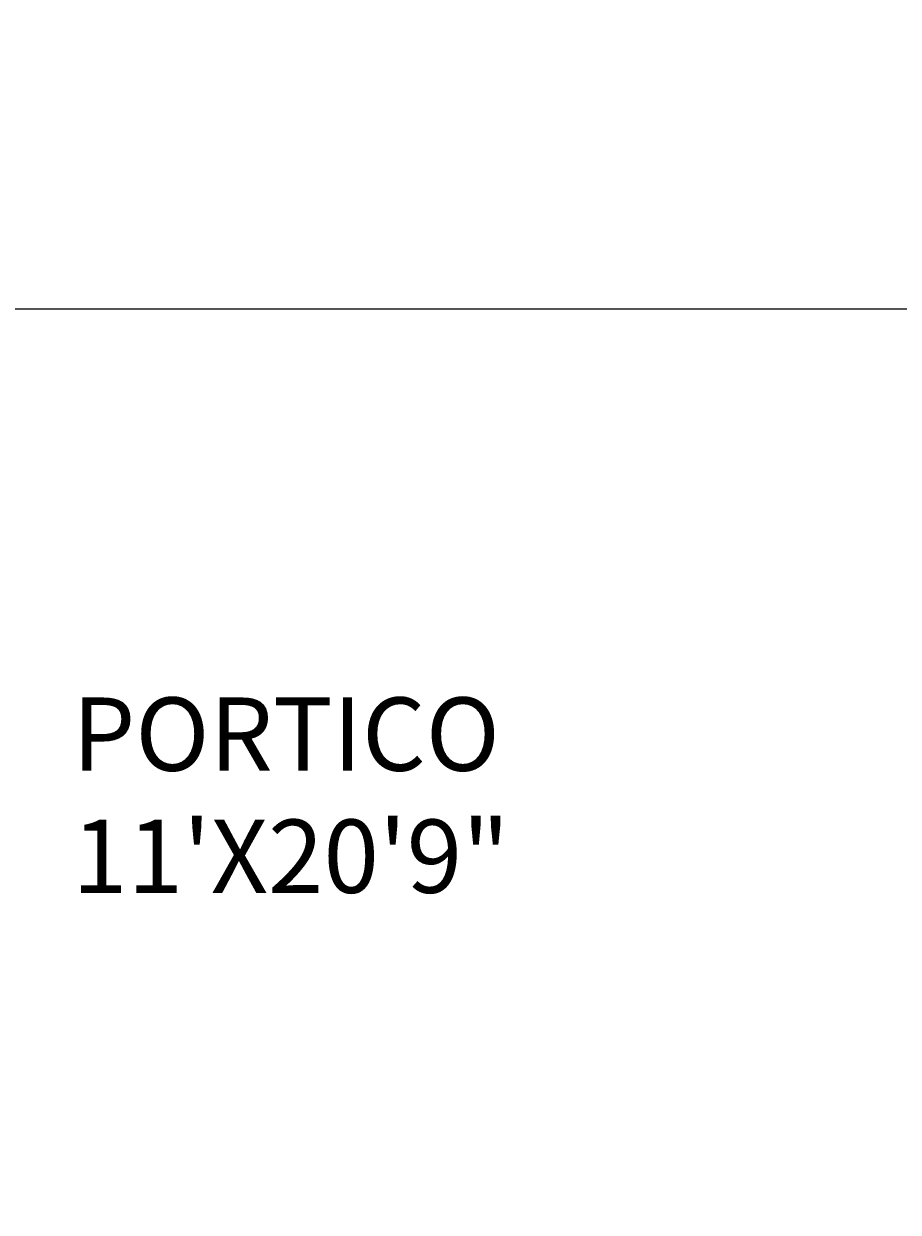
# Model space of a CAD drawing. Units: inches. Extents: x -4347 to -3836, y 955 to 1521.
# Tile 6 of 11: x -4072 to -4001, y 1023 to 1120. Entities that reach past the tile are written whole.
import ezdxf

# ---------------------------------------------------------------- set-up
doc = ezdxf.new("R2010")
doc.units = ezdxf.units.IN
doc.header["$MEASUREMENT"] = 0
doc.layers.add('A-ANNO-DIMS', color=2, linetype='Continuous', lineweight=18)
doc.layers.add('A-AREA-IDEN', color=7, linetype='Continuous', lineweight=18)
doc.styles.get("Standard").update_dxf_attribs({"font": 'arial.ttf'})
doc.dimstyles.get("Standard").update_dxf_attribs({"dimtxt": 0.18, "dimasz": 0.18, "dimexe": 0.18, "dimexo": 0.0625, "dimgap": 0.09, "dimtad": 0, "dimtih": 1, "dimtoh": 1, "dimdec": 0, "dimzin": 0, "dimdsep": 46, "dimlunit": 3, "dimtxsty": 'Standard', "dimcen": 0.09, "dimadec": 0, "dimazin": 0, "dimtfac": 1, "dimtdec": 0, "dimtofl": 0, "dimtmove": 0, "dimatfit": 3, "dimfxl": 1, "dimtolj": 1, "dimtzin": 0, "dimarcsym": 0})

# ---------------------------------------------------------------- blocks, each defined once
blk = doc.blocks.new('*D47')
at = {"layer": 'A-ANNO-DIMS', "color": 0, "lineweight": -2, "transparency": 16777216}
for p, q in [((-4120.58, 1288.726), (-4120.58, 966.959)), ((-3940.58, 1288.726), (-3940.58, 966.959)), ((-4120.4, 967.139), (-4030.97, 967.139)), ((-3940.76, 967.139), (-4030.189, 967.139))]:
    blk.add_line(p, q, dxfattribs=at)
at = {"layer": 'A-ANNO-DIMS', "color": 0, "transparency": 16777216}
for points in [[(-4120.4, 967.169), (-4120.4, 967.109), (-4120.58, 967.139)], [(-3940.76, 967.169), (-3940.76, 967.109), (-3940.58, 967.139)]]:
    blk.add_solid(points, dxfattribs=at)
at = {"layer": 'Defpoints', "color": 0, "transparency": 16777216}
for p in [(-4120.58, 1288.789), (-3940.58, 1288.789), (-3940.58, 967.139)]:
    blk.add_point(p, dxfattribs=at)
at = {"layer": 'A-ANNO-DIMS', "color": 0, "transparency": 16777216, "insert": (-4030.58, 967.139), "char_height": 0.18, "attachment_point": 5}
blk.add_mtext('\\A1;15\'-0"', dxfattribs=at)
blk = doc.blocks.new('*D54')
at = {"layer": 'A-ANNO-DIMS', "color": 0, "lineweight": -2, "transparency": 16777216}
for p, q in [((-3997.757, 1126.789), (-4346.41, 1126.789)), ((-4346.23, 1126.609), (-4346.23, 1111.971)), ((-4346.23, 1096.969), (-4346.23, 1111.607)), ((-3997.757, 1096.789), (-4346.41, 1096.789))]:
    blk.add_line(p, q, dxfattribs=at)
at = {"layer": 'A-ANNO-DIMS', "color": 0, "transparency": 16777216}
for points in [[(-4346.26, 1126.609), (-4346.2, 1126.609), (-4346.23, 1126.789)], [(-4346.26, 1096.969), (-4346.2, 1096.969), (-4346.23, 1096.789)]]:
    blk.add_solid(points, dxfattribs=at)
at = {"layer": 'Defpoints', "color": 0, "transparency": 16777216}
for p in [(-4346.23, 1126.789), (-3997.694, 1126.789), (-3997.694, 1096.789)]:
    blk.add_point(p, dxfattribs=at)
at = {"layer": 'A-ANNO-DIMS', "color": 0, "transparency": 16777216, "insert": (-4346.23, 1111.789), "char_height": 0.18, "attachment_point": 5}
blk.add_mtext('\\A1;2\'-6"', dxfattribs=at)

msp = doc.modelspace()

# ---------------------------------------------------------------- texts
at = {"layer": 'A-AREA-IDEN', "insert": (-4068.458, 1065.009), "char_height": 6, "attachment_point": 1}
msp.add_mtext('PORTICO\\P11\'X20\'9"', dxfattribs=at)

# ---------------------------------------------------------------- dimensions: what is measured, and where the dimension line sits
at = {"layer": 'A-ANNO-DIMS'}
dim = msp.add_linear_dim(base=(-3940.58, 967.139), p1=(-4120.58, 1288.789), p2=(-3940.58, 1288.789), dimstyle='Standard', override={"dimdec": 1, "dimlfac": 1, "dimrnd": 0, "dimzin": 1, "dimdsep": 46, "dimlunit": 4, "dimfrac": 2}, dxfattribs=at)
dim.commit()
dim.dimension.update_dxf_attribs({"geometry": '*D47', "text_midpoint": (-4030.58, 967.139)})
dim = msp.add_linear_dim(base=(-4346.23, 1126.789), p1=(-3997.694, 1096.789), p2=(-3997.694, 1126.789), angle=90, dimstyle='Standard', override={"dimdec": 1, "dimlfac": 1, "dimrnd": 0, "dimzin": 1, "dimdsep": 46, "dimlunit": 4, "dimfrac": 2}, dxfattribs=at)
dim.commit()
dim.dimension.update_dxf_attribs({"geometry": '*D54', "text_midpoint": (-4346.23, 1111.789)})

doc.saveas('drawing.dxf')
